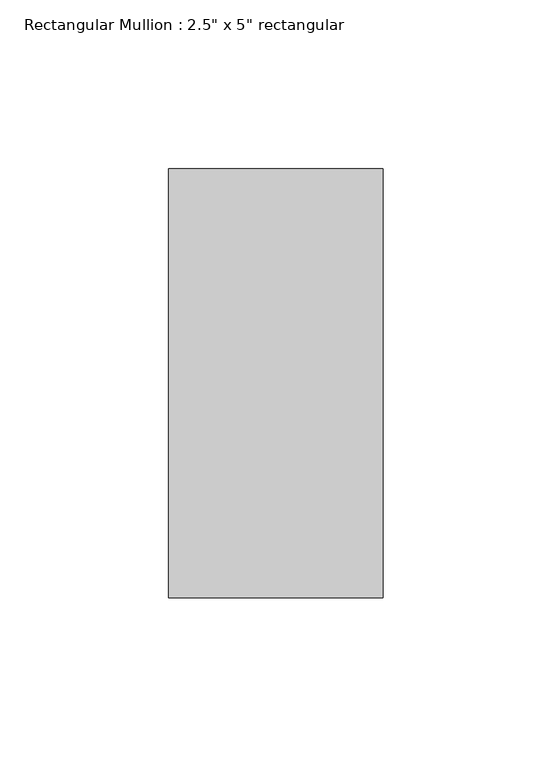
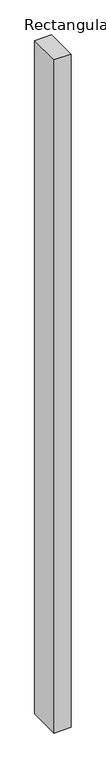
"""IFC4 building model written with IfcOpenShell, lengths in millimetres: member geometry."""

from ifc_helpers import new_model, si_unit, frame, origin, place, context, project, spatial, polyline, outline, extrude, source, transform, mapped, element, save


def member_9661c287(model_context):
    return source(origin(), model_context, "Body", "SweptSolid", [
        extrude(outline(polyline([(31.75, 63.5), (31.75, -63.5), (-31.75, -63.5), (-31.75, 63.5), (31.75, 63.5)])), frame((0.0, 0.0, -2667.0), z_axis=(0.0, 0.0, 1.0), x_axis=(1.0, 0.0, 0.0)), (0.0, 0.0, 1.0), 2667.0),
    ])


if __name__ == "__main__":
    model = new_model("IFC4")
    model_context = context("Model", 3, world=origin())
    ifc_project = project(units=[si_unit("LENGTHUNIT", "METRE", prefix="MILLI")], contexts=[model_context])
    site = spatial("IfcSite", under=ifc_project)
    building = spatial("IfcBuilding", under=site)
    placement = place(None, origin())
    member_shape = member_9661c287(model_context)
    element("IfcMember", 1, ObjectType="Rectangular Mullion : 2.5\" x 5\" rectangular", at=placement, inside=building, context=model_context, shape_type="MappedRepresentation", body=[
        mapped(member_shape, transform((0.0, 0.0, 0.0), x_axis=(1.0, 0.0, 0.0), y_axis=(0.0, 1.0, 0.0), z_axis=(0.0, 0.0, 1.0))),
    ])
    save(model, "model.ifc")

# Revit data of these elements
# Type "Rectangular Mullion : 2.5\" x 5\" rectangular"
#   built-in parameter 1007304 = 0.416667 (stored number, unit not read)
#   built-in parameter 1007301 = 0.104167 (stored number, unit not read)
#   built-in parameter 1007300 = 0.104167 (stored number, unit not read)
